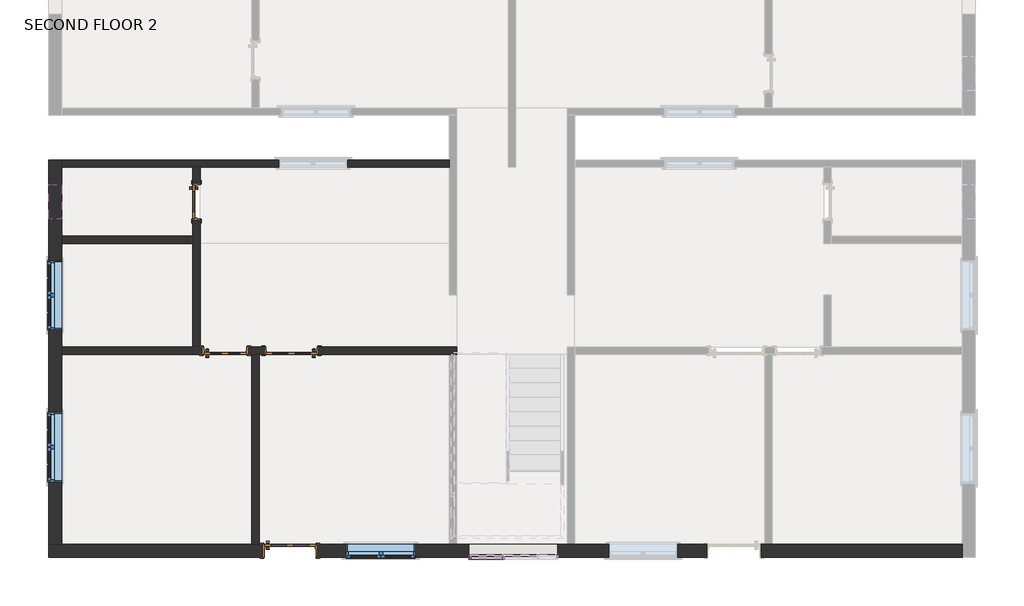
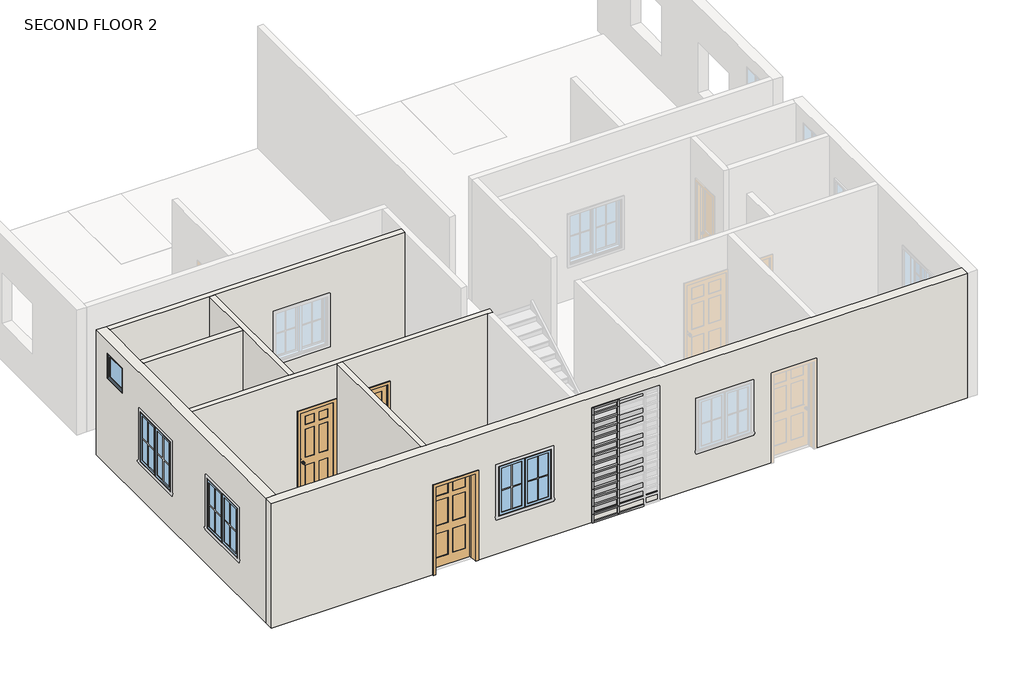
# One storey, part 1 of 4: 44 members, 21 plates, 7 walls, 4 doors, 4 windows.
"""IFC4 building model written with IfcOpenShell, lengths in millimetres."""

from ifc_helpers import new_model, si_unit, frame, origin, place, context, project, spatial, polyline, outline, extrude, faceted_brep, transform, mapped, element, save
from components import door_e337afa5, door_3b50870b, door_d86b6c54, door_03e3dfb5, member_56b223d9, member_a59c64b1, member_fa69921b, member_a67f877f, member_6a7c88b6, member_dc11c383, member_ff422208, system_panel_glazed_844a74e3, system_panel_glazed_a39216e9, system_panel_glazed_b3845325, system_panel_glazed_23b8b45c, system_panel_glazed_26c33eb0, system_panel_glazed_afc0885c, window_80340324, window_9200f5ac

model = new_model("IFC4")

# Units and contexts
model_context = context("Model", 3, world=origin())
ifc_project = project(units=[si_unit("LENGTHUNIT", "METRE", prefix="MILLI")], contexts=[model_context])

# Site, building, storey
site = spatial("IfcSite", under=ifc_project)
building = spatial("IfcBuilding", under=site)
storey = spatial("IfcBuildingStorey", under=building, Name="SECOND FLOOR 2", Elevation=6343.9725604)

# Doors
placement = place(None, origin())
door_shape = door_e337afa5(model_context)
element("IfcDoor", 1, ObjectType="Door-Interior-Single-2_Panel-Wood : 24\" x 84\"", at=placement, inside=storey, context=model_context, shape_type="MappedRepresentation", body=[
    mapped(door_shape, transform((-9830.0887331, -1548.6593836, 6343.9725604), x_axis=(0.0, -1.0, 0.0), y_axis=(1.0, 0.0, 0.0), z_axis=(0.0, 0.0, 1.0))),
])
door_2_shape = door_3b50870b(model_context)
element("IfcDoor", 2, ObjectType="Door-Interior-Single-6_Panel-Wood : 30\" x 84\"", at=placement, inside=storey, context=model_context, shape_type="MappedRepresentation", body=[
    mapped(door_2_shape, transform((-9318.9137331, -4180.7343836, 6343.9725604), x_axis=(1.0, 0.0, 0.0), y_axis=(0.0, 1.0, 0.0), z_axis=(0.0, 0.0, 1.0))),
])
door_3_shape = door_d86b6c54(model_context)
element("IfcDoor", 3, ObjectType="Door-Interior-Single-6_Panel-Wood : 36\" x 84\"", at=placement, inside=storey, context=model_context, shape_type="MappedRepresentation", body=[
    mapped(door_3_shape, transform((-8175.9137331, -7704.9843836, 6343.9725604), x_axis=(1.0, 0.0, 0.0), y_axis=(0.0, 1.0, 0.0), z_axis=(0.0, 0.0, 1.0))),
])
door_4_shape = door_03e3dfb5(model_context)
element("IfcDoor", 4, ObjectType="Door-Interior-Single-6_Panel-Wood : 36\" x 84\"", at=placement, inside=storey, context=model_context, shape_type="MappedRepresentation", body=[
    mapped(door_4_shape, transform((-8150.5137331, -4180.7343836, 6343.9725604), x_axis=(-1.0, 0.0, 0.0), y_axis=(0.0, -1.0, 0.0), z_axis=(0.0, 0.0, 1.0))),
])

# Members
member_shape = member_56b223d9(model_context)
element("IfcMember", 5, ObjectType="Rectangular Mullion : 1.5\" x 2.5\" rectangular", at=placement, inside=storey, context=model_context, shape_type="MappedRepresentation", body=[
    mapped(member_shape, transform((-4416.6334597, -7822.4593836, 6343.9725604), x_axis=(1.0, 0.0, 0.0), y_axis=(0.0, -1.0, 0.0), z_axis=(0.0, 0.0, -1.0))),
])
element("IfcMember", 6, ObjectType="Rectangular Mullion : 1.5\" x 2.5\" rectangular", at=placement, inside=storey, context=model_context, shape_type="MappedRepresentation", body=[
    mapped(member_shape, transform((-4416.6334597, -7822.4593836, 6547.1725604), x_axis=(1.0, 0.0, 0.0), y_axis=(0.0, -1.0, 0.0), z_axis=(0.0, 0.0, -1.0))),
])
element("IfcMember", 7, ObjectType="Rectangular Mullion : 1.5\" x 2.5\" rectangular", at=placement, inside=storey, context=model_context, shape_type="MappedRepresentation", body=[
    mapped(member_shape, transform((-4416.6334597, -7822.4593836, 6750.3725604), x_axis=(1.0, 0.0, 0.0), y_axis=(0.0, -1.0, 0.0), z_axis=(0.0, 0.0, -1.0))),
])
element("IfcMember", 8, ObjectType="Rectangular Mullion : 1.5\" x 2.5\" rectangular", at=placement, inside=storey, context=model_context, shape_type="MappedRepresentation", body=[
    mapped(member_shape, transform((-4416.6334597, -7822.4593836, 6953.5725604), x_axis=(1.0, 0.0, 0.0), y_axis=(0.0, -1.0, 0.0), z_axis=(0.0, 0.0, -1.0))),
])
element("IfcMember", 9, ObjectType="Rectangular Mullion : 1.5\" x 2.5\" rectangular", at=placement, inside=storey, context=model_context, shape_type="MappedRepresentation", body=[
    mapped(member_shape, transform((-4416.6334597, -7822.4593836, 7156.7725604), x_axis=(1.0, 0.0, 0.0), y_axis=(0.0, -1.0, 0.0), z_axis=(0.0, 0.0, -1.0))),
])
element("IfcMember", 10, ObjectType="Rectangular Mullion : 1.5\" x 2.5\" rectangular", at=placement, inside=storey, context=model_context, shape_type="MappedRepresentation", body=[
    mapped(member_shape, transform((-4416.6334597, -7822.4593836, 7359.9725604), x_axis=(1.0, 0.0, 0.0), y_axis=(0.0, -1.0, 0.0), z_axis=(0.0, 0.0, -1.0))),
])
element("IfcMember", 11, ObjectType="Rectangular Mullion : 1.5\" x 2.5\" rectangular", at=placement, inside=storey, context=model_context, shape_type="MappedRepresentation", body=[
    mapped(member_shape, transform((-4416.6334597, -7822.4593836, 7563.1725604), x_axis=(1.0, 0.0, 0.0), y_axis=(0.0, -1.0, 0.0), z_axis=(0.0, 0.0, -1.0))),
])
element("IfcMember", 12, ObjectType="Rectangular Mullion : 1.5\" x 2.5\" rectangular", at=placement, inside=storey, context=model_context, shape_type="MappedRepresentation", body=[
    mapped(member_shape, transform((-4416.6334597, -7822.4593836, 7766.3725604), x_axis=(1.0, 0.0, 0.0), y_axis=(0.0, -1.0, 0.0), z_axis=(0.0, 0.0, -1.0))),
])
element("IfcMember", 13, ObjectType="Rectangular Mullion : 1.5\" x 2.5\" rectangular", at=placement, inside=storey, context=model_context, shape_type="MappedRepresentation", body=[
    mapped(member_shape, transform((-4416.6334597, -7822.4593836, 7969.5725604), x_axis=(1.0, 0.0, 0.0), y_axis=(0.0, -1.0, 0.0), z_axis=(0.0, 0.0, -1.0))),
])
element("IfcMember", 14, ObjectType="Rectangular Mullion : 1.5\" x 2.5\" rectangular", at=placement, inside=storey, context=model_context, shape_type="MappedRepresentation", body=[
    mapped(member_shape, transform((-4416.6334597, -7822.4593836, 8172.7725604), x_axis=(1.0, 0.0, 0.0), y_axis=(0.0, -1.0, 0.0), z_axis=(0.0, 0.0, -1.0))),
])
element("IfcMember", 15, ObjectType="Rectangular Mullion : 1.5\" x 2.5\" rectangular", at=placement, inside=storey, context=model_context, shape_type="MappedRepresentation", body=[
    mapped(member_shape, transform((-4416.6334597, -7822.4593836, 8375.9725604), x_axis=(1.0, 0.0, 0.0), y_axis=(0.0, -1.0, 0.0), z_axis=(0.0, 0.0, -1.0))),
])
element("IfcMember", 16, ObjectType="Rectangular Mullion : 1.5\" x 2.5\" rectangular", at=placement, inside=storey, context=model_context, shape_type="MappedRepresentation", body=[
    mapped(member_shape, transform((-4416.6334597, -7822.4593836, 8579.1725604), x_axis=(1.0, 0.0, 0.0), y_axis=(0.0, -1.0, 0.0), z_axis=(0.0, 0.0, -1.0))),
])
element("IfcMember", 17, ObjectType="Rectangular Mullion : 1.5\" x 2.5\" rectangular", at=placement, inside=storey, context=model_context, shape_type="MappedRepresentation", body=[
    mapped(member_shape, transform((-4416.6334597, -7822.4593836, 8782.3725604), x_axis=(1.0, 0.0, 0.0), y_axis=(0.0, -1.0, 0.0), z_axis=(0.0, 0.0, -1.0))),
])
member_2_shape = member_a59c64b1(model_context)
element("IfcMember", 18, ObjectType="Rectangular Mullion : 1.5\" x 2.5\" rectangular", at=placement, inside=storey, context=model_context, shape_type="MappedRepresentation", body=[
    mapped(member_2_shape, transform((-4416.6334597, -7822.4593836, 8985.5725604), x_axis=(1.0, 0.0, 0.0), y_axis=(0.0, -1.0, 0.0), z_axis=(0.0, 0.0, -1.0))),
])
member_3_shape = member_fa69921b(model_context)
element("IfcMember", 19, ObjectType="Rectangular Mullion : 1.5\" x 2.5\" rectangular", at=placement, inside=storey, context=model_context, shape_type="MappedRepresentation", body=[
    mapped(member_3_shape, transform((-4435.6834597, -7822.4593836, 9151.3551755), x_axis=(0.0, 0.0, 1.0), y_axis=(0.0, -1.0, 0.0), z_axis=(1.0, 0.0, 0.0))),
])
element("IfcMember", 20, ObjectType="Rectangular Mullion : 1.5\" x 2.5\" rectangular", at=placement, inside=storey, context=model_context, shape_type="MappedRepresentation", body=[
    mapped(member_3_shape, transform((-4988.13346, -7822.4593836, 6343.9725604), x_axis=(0.0, 0.0, -1.0), y_axis=(0.0, -1.0, 0.0), z_axis=(-1.0, 0.0, 0.0))),
])
member_4_shape = member_a67f877f(model_context)
element("IfcMember", 21, ObjectType="Rectangular Mullion : 1.5\" x 2.5\" rectangular", at=placement, inside=storey, context=model_context, shape_type="MappedRepresentation", body=[
    mapped(member_4_shape, transform((-4397.5834597, -7822.4593836, 6343.9725604), x_axis=(0.0, 0.0, -1.0), y_axis=(0.0, -1.0, 0.0), z_axis=(-1.0, 0.0, 0.0))),
])
member_5_shape = member_6a7c88b6(model_context)
element("IfcMember", 22, ObjectType="Rectangular Mullion : 1.5\" x 2.5\" rectangular", at=placement, inside=storey, context=model_context, shape_type="MappedRepresentation", body=[
    mapped(member_5_shape, transform((-4435.6834597, -7822.4593836, 6547.1725604), x_axis=(0.0, 0.0, 1.0), y_axis=(0.0, -1.0, 0.0), z_axis=(1.0, 0.0, 0.0))),
])
element("IfcMember", 23, ObjectType="Rectangular Mullion : 1.5\" x 2.5\" rectangular", at=placement, inside=storey, context=model_context, shape_type="MappedRepresentation", body=[
    mapped(member_5_shape, transform((-4435.6834597, -7822.4593836, 6750.3725604), x_axis=(0.0, 0.0, 1.0), y_axis=(0.0, -1.0, 0.0), z_axis=(1.0, 0.0, 0.0))),
])
element("IfcMember", 24, ObjectType="Rectangular Mullion : 1.5\" x 2.5\" rectangular", at=placement, inside=storey, context=model_context, shape_type="MappedRepresentation", body=[
    mapped(member_5_shape, transform((-4435.6834597, -7822.4593836, 6953.5725604), x_axis=(0.0, 0.0, 1.0), y_axis=(0.0, -1.0, 0.0), z_axis=(1.0, 0.0, 0.0))),
])
element("IfcMember", 25, ObjectType="Rectangular Mullion : 1.5\" x 2.5\" rectangular", at=placement, inside=storey, context=model_context, shape_type="MappedRepresentation", body=[
    mapped(member_5_shape, transform((-4435.6834597, -7822.4593836, 7156.7725604), x_axis=(0.0, 0.0, 1.0), y_axis=(0.0, -1.0, 0.0), z_axis=(1.0, 0.0, 0.0))),
])
element("IfcMember", 26, ObjectType="Rectangular Mullion : 1.5\" x 2.5\" rectangular", at=placement, inside=storey, context=model_context, shape_type="MappedRepresentation", body=[
    mapped(member_5_shape, transform((-4435.6834597, -7822.4593836, 7359.9725604), x_axis=(0.0, 0.0, 1.0), y_axis=(0.0, -1.0, 0.0), z_axis=(1.0, 0.0, 0.0))),
])
element("IfcMember", 27, ObjectType="Rectangular Mullion : 1.5\" x 2.5\" rectangular", at=placement, inside=storey, context=model_context, shape_type="MappedRepresentation", body=[
    mapped(member_5_shape, transform((-4435.6834597, -7822.4593836, 7563.1725604), x_axis=(0.0, 0.0, 1.0), y_axis=(0.0, -1.0, 0.0), z_axis=(1.0, 0.0, 0.0))),
])
element("IfcMember", 28, ObjectType="Rectangular Mullion : 1.5\" x 2.5\" rectangular", at=placement, inside=storey, context=model_context, shape_type="MappedRepresentation", body=[
    mapped(member_5_shape, transform((-4435.6834597, -7822.4593836, 7766.3725604), x_axis=(0.0, 0.0, 1.0), y_axis=(0.0, -1.0, 0.0), z_axis=(1.0, 0.0, 0.0))),
])
element("IfcMember", 29, ObjectType="Rectangular Mullion : 1.5\" x 2.5\" rectangular", at=placement, inside=storey, context=model_context, shape_type="MappedRepresentation", body=[
    mapped(member_5_shape, transform((-4435.6834597, -7822.4593836, 7969.5725604), x_axis=(0.0, 0.0, 1.0), y_axis=(0.0, -1.0, 0.0), z_axis=(1.0, 0.0, 0.0))),
])
element("IfcMember", 30, ObjectType="Rectangular Mullion : 1.5\" x 2.5\" rectangular", at=placement, inside=storey, context=model_context, shape_type="MappedRepresentation", body=[
    mapped(member_5_shape, transform((-4435.6834597, -7822.4593836, 8172.7725604), x_axis=(0.0, 0.0, 1.0), y_axis=(0.0, -1.0, 0.0), z_axis=(1.0, 0.0, 0.0))),
])
element("IfcMember", 31, ObjectType="Rectangular Mullion : 1.5\" x 2.5\" rectangular", at=placement, inside=storey, context=model_context, shape_type="MappedRepresentation", body=[
    mapped(member_5_shape, transform((-4435.6834597, -7822.4593836, 8375.9725604), x_axis=(0.0, 0.0, 1.0), y_axis=(0.0, -1.0, 0.0), z_axis=(1.0, 0.0, 0.0))),
])
element("IfcMember", 32, ObjectType="Rectangular Mullion : 1.5\" x 2.5\" rectangular", at=placement, inside=storey, context=model_context, shape_type="MappedRepresentation", body=[
    mapped(member_5_shape, transform((-4435.6834597, -7822.4593836, 8579.1725604), x_axis=(0.0, 0.0, 1.0), y_axis=(0.0, -1.0, 0.0), z_axis=(1.0, 0.0, 0.0))),
])
element("IfcMember", 33, ObjectType="Rectangular Mullion : 1.5\" x 2.5\" rectangular", at=placement, inside=storey, context=model_context, shape_type="MappedRepresentation", body=[
    mapped(member_5_shape, transform((-4435.6834597, -7822.4593836, 8782.3725604), x_axis=(0.0, 0.0, 1.0), y_axis=(0.0, -1.0, 0.0), z_axis=(1.0, 0.0, 0.0))),
])
element("IfcMember", 34, ObjectType="Rectangular Mullion : 1.5\" x 2.5\" rectangular", at=placement, inside=storey, context=model_context, shape_type="MappedRepresentation", body=[
    mapped(member_5_shape, transform((-4435.6834597, -7822.4593836, 8985.5725604), x_axis=(0.0, 0.0, 1.0), y_axis=(0.0, -1.0, 0.0), z_axis=(1.0, 0.0, 0.0))),
])
member_6_shape = member_dc11c383(model_context)
element("IfcMember", 35, ObjectType="Rectangular Mullion : 1.5\" x 2.5\" rectangular", at=placement, inside=storey, context=model_context, shape_type="MappedRepresentation", body=[
    mapped(member_6_shape, transform((-5026.23346, -7822.4593836, 9151.3551755), x_axis=(-1.0, 0.0, 0.0), y_axis=(0.0, -1.0, 0.0), z_axis=(0.0, 0.0, 1.0))),
])
member_7_shape = member_ff422208(model_context)
element("IfcMember", 36, ObjectType="Rectangular Mullion : 1.5\" x 2.5\" rectangular", at=placement, inside=storey, context=model_context, shape_type="MappedRepresentation", body=[
    mapped(member_7_shape, transform((-5026.23346, -7822.4593836, 6547.1725604), x_axis=(-1.0, 0.0, 0.0), y_axis=(0.0, -1.0, 0.0), z_axis=(0.0, 0.0, 1.0))),
])
element("IfcMember", 37, ObjectType="Rectangular Mullion : 1.5\" x 2.5\" rectangular", at=placement, inside=storey, context=model_context, shape_type="MappedRepresentation", body=[
    mapped(member_7_shape, transform((-5026.23346, -7822.4593836, 6750.3725604), x_axis=(-1.0, 0.0, 0.0), y_axis=(0.0, -1.0, 0.0), z_axis=(0.0, 0.0, 1.0))),
])
element("IfcMember", 38, ObjectType="Rectangular Mullion : 1.5\" x 2.5\" rectangular", at=placement, inside=storey, context=model_context, shape_type="MappedRepresentation", body=[
    mapped(member_7_shape, transform((-5026.23346, -7822.4593836, 6953.5725604), x_axis=(-1.0, 0.0, 0.0), y_axis=(0.0, -1.0, 0.0), z_axis=(0.0, 0.0, 1.0))),
])
element("IfcMember", 39, ObjectType="Rectangular Mullion : 1.5\" x 2.5\" rectangular", at=placement, inside=storey, context=model_context, shape_type="MappedRepresentation", body=[
    mapped(member_7_shape, transform((-5026.23346, -7822.4593836, 7156.7725604), x_axis=(-1.0, 0.0, 0.0), y_axis=(0.0, -1.0, 0.0), z_axis=(0.0, 0.0, 1.0))),
])
element("IfcMember", 40, ObjectType="Rectangular Mullion : 1.5\" x 2.5\" rectangular", at=placement, inside=storey, context=model_context, shape_type="MappedRepresentation", body=[
    mapped(member_7_shape, transform((-5026.23346, -7822.4593836, 7359.9725604), x_axis=(-1.0, 0.0, 0.0), y_axis=(0.0, -1.0, 0.0), z_axis=(0.0, 0.0, 1.0))),
])
element("IfcMember", 41, ObjectType="Rectangular Mullion : 1.5\" x 2.5\" rectangular", at=placement, inside=storey, context=model_context, shape_type="MappedRepresentation", body=[
    mapped(member_7_shape, transform((-5026.23346, -7822.4593836, 7563.1725604), x_axis=(-1.0, 0.0, 0.0), y_axis=(0.0, -1.0, 0.0), z_axis=(0.0, 0.0, 1.0))),
])
element("IfcMember", 42, ObjectType="Rectangular Mullion : 1.5\" x 2.5\" rectangular", at=placement, inside=storey, context=model_context, shape_type="MappedRepresentation", body=[
    mapped(member_7_shape, transform((-5026.23346, -7822.4593836, 7766.3725604), x_axis=(-1.0, 0.0, 0.0), y_axis=(0.0, -1.0, 0.0), z_axis=(0.0, 0.0, 1.0))),
])
element("IfcMember", 43, ObjectType="Rectangular Mullion : 1.5\" x 2.5\" rectangular", at=placement, inside=storey, context=model_context, shape_type="MappedRepresentation", body=[
    mapped(member_7_shape, transform((-5026.23346, -7822.4593836, 7969.5725604), x_axis=(-1.0, 0.0, 0.0), y_axis=(0.0, -1.0, 0.0), z_axis=(0.0, 0.0, 1.0))),
])
element("IfcMember", 44, ObjectType="Rectangular Mullion : 1.5\" x 2.5\" rectangular", at=placement, inside=storey, context=model_context, shape_type="MappedRepresentation", body=[
    mapped(member_7_shape, transform((-5026.23346, -7822.4593836, 8172.7725604), x_axis=(-1.0, 0.0, 0.0), y_axis=(0.0, -1.0, 0.0), z_axis=(0.0, 0.0, 1.0))),
])
element("IfcMember", 45, ObjectType="Rectangular Mullion : 1.5\" x 2.5\" rectangular", at=placement, inside=storey, context=model_context, shape_type="MappedRepresentation", body=[
    mapped(member_7_shape, transform((-5026.23346, -7822.4593836, 8375.9725604), x_axis=(-1.0, 0.0, 0.0), y_axis=(0.0, -1.0, 0.0), z_axis=(0.0, 0.0, 1.0))),
])
element("IfcMember", 46, ObjectType="Rectangular Mullion : 1.5\" x 2.5\" rectangular", at=placement, inside=storey, context=model_context, shape_type="MappedRepresentation", body=[
    mapped(member_7_shape, transform((-5026.23346, -7822.4593836, 8579.1725604), x_axis=(-1.0, 0.0, 0.0), y_axis=(0.0, -1.0, 0.0), z_axis=(0.0, 0.0, 1.0))),
])
element("IfcMember", 47, ObjectType="Rectangular Mullion : 1.5\" x 2.5\" rectangular", at=placement, inside=storey, context=model_context, shape_type="MappedRepresentation", body=[
    mapped(member_7_shape, transform((-5026.23346, -7822.4593836, 8782.3725604), x_axis=(-1.0, 0.0, 0.0), y_axis=(0.0, -1.0, 0.0), z_axis=(0.0, 0.0, 1.0))),
])
element("IfcMember", 48, ObjectType="Rectangular Mullion : 1.5\" x 2.5\" rectangular", at=placement, inside=storey, context=model_context, shape_type="MappedRepresentation", body=[
    mapped(member_7_shape, transform((-5026.23346, -7822.4593836, 8985.5725604), x_axis=(-1.0, 0.0, 0.0), y_axis=(0.0, -1.0, 0.0), z_axis=(0.0, 0.0, 1.0))),
])

# Plates
system_panel_glazed_shape = system_panel_glazed_844a74e3(model_context)
element("IfcPlate", 49, ObjectType="System Panel : Glazed", at=placement, inside=storey, context=model_context, shape_type="MappedRepresentation", body=[
    mapped(system_panel_glazed_shape, transform((-4711.9084599, -7822.4593836, 6382.0725604), x_axis=(1.0, 0.0, 0.0), y_axis=(0.0, 1.0, 0.0), z_axis=(0.0, 0.0, 1.0))),
])
system_panel_glazed_2_shape = system_panel_glazed_a39216e9(model_context)
element("IfcPlate", 50, ObjectType="System Panel : Glazed", at=placement, inside=storey, context=model_context, shape_type="MappedRepresentation", body=[
    mapped(system_panel_glazed_2_shape, transform((-4111.8334597, -7822.4593836, 6382.0725604), x_axis=(1.0, 0.0, 0.0), y_axis=(0.0, 1.0, 0.0), z_axis=(0.0, 0.0, 1.0))),
])
system_panel_glazed_3_shape = system_panel_glazed_b3845325(model_context)
element("IfcPlate", 51, ObjectType="System Panel : Glazed", at=placement, inside=storey, context=model_context, shape_type="MappedRepresentation", body=[
    mapped(system_panel_glazed_3_shape, transform((-4711.9084599, -7822.4593836, 6566.2225604), x_axis=(1.0, 0.0, 0.0), y_axis=(0.0, 1.0, 0.0), z_axis=(0.0, 0.0, 1.0))),
])
element("IfcPlate", 52, ObjectType="System Panel : Glazed", at=placement, inside=storey, context=model_context, shape_type="MappedRepresentation", body=[
    mapped(system_panel_glazed_3_shape, transform((-4711.9084599, -7822.4593836, 6769.4225604), x_axis=(1.0, 0.0, 0.0), y_axis=(0.0, 1.0, 0.0), z_axis=(0.0, 0.0, 1.0))),
])
element("IfcPlate", 53, ObjectType="System Panel : Glazed", at=placement, inside=storey, context=model_context, shape_type="MappedRepresentation", body=[
    mapped(system_panel_glazed_3_shape, transform((-4711.9084599, -7822.4593836, 7175.8225604), x_axis=(1.0, 0.0, 0.0), y_axis=(0.0, 1.0, 0.0), z_axis=(0.0, 0.0, 1.0))),
])
element("IfcPlate", 54, ObjectType="System Panel : Glazed", at=placement, inside=storey, context=model_context, shape_type="MappedRepresentation", body=[
    mapped(system_panel_glazed_3_shape, transform((-4711.9084599, -7822.4593836, 7379.0225604), x_axis=(1.0, 0.0, 0.0), y_axis=(0.0, 1.0, 0.0), z_axis=(0.0, 0.0, 1.0))),
])
element("IfcPlate", 55, ObjectType="System Panel : Glazed", at=placement, inside=storey, context=model_context, shape_type="MappedRepresentation", body=[
    mapped(system_panel_glazed_3_shape, transform((-4711.9084599, -7822.4593836, 7785.4225604), x_axis=(1.0, 0.0, 0.0), y_axis=(0.0, 1.0, 0.0), z_axis=(0.0, 0.0, 1.0))),
])
element("IfcPlate", 56, ObjectType="System Panel : Glazed", at=placement, inside=storey, context=model_context, shape_type="MappedRepresentation", body=[
    mapped(system_panel_glazed_3_shape, transform((-4711.9084599, -7822.4593836, 7988.6225604), x_axis=(1.0, 0.0, 0.0), y_axis=(0.0, 1.0, 0.0), z_axis=(0.0, 0.0, 1.0))),
])
element("IfcPlate", 57, ObjectType="System Panel : Glazed", at=placement, inside=storey, context=model_context, shape_type="MappedRepresentation", body=[
    mapped(system_panel_glazed_3_shape, transform((-4711.9084599, -7822.4593836, 8395.0225604), x_axis=(1.0, 0.0, 0.0), y_axis=(0.0, 1.0, 0.0), z_axis=(0.0, 0.0, 1.0))),
])
element("IfcPlate", 58, ObjectType="System Panel : Glazed", at=placement, inside=storey, context=model_context, shape_type="MappedRepresentation", body=[
    mapped(system_panel_glazed_3_shape, transform((-4711.9084599, -7822.4593836, 8598.2225604), x_axis=(1.0, 0.0, 0.0), y_axis=(0.0, 1.0, 0.0), z_axis=(0.0, 0.0, 1.0))),
])
element("IfcPlate", 59, ObjectType="System Panel : Glazed", at=placement, inside=storey, context=model_context, shape_type="MappedRepresentation", body=[
    mapped(system_panel_glazed_3_shape, transform((-4711.9084599, -7822.4593836, 6972.6225604), x_axis=(1.0, 0.0, 0.0), y_axis=(0.0, 1.0, 0.0), z_axis=(0.0, 0.0, 1.0))),
])
system_panel_glazed_4_shape = system_panel_glazed_23b8b45c(model_context)
element("IfcPlate", 60, ObjectType="System Panel : Glazed", at=placement, inside=storey, context=model_context, shape_type="MappedRepresentation", body=[
    mapped(system_panel_glazed_4_shape, transform((-4111.8334597, -7822.4593836, 6566.2225604), x_axis=(1.0, 0.0, 0.0), y_axis=(0.0, 1.0, 0.0), z_axis=(0.0, 0.0, 1.0))),
])
element("IfcPlate", 61, ObjectType="System Panel : Glazed", at=placement, inside=storey, context=model_context, shape_type="MappedRepresentation", body=[
    mapped(system_panel_glazed_4_shape, transform((-4111.8334597, -7822.4593836, 6769.4225604), x_axis=(1.0, 0.0, 0.0), y_axis=(0.0, 1.0, 0.0), z_axis=(0.0, 0.0, 1.0))),
])
element("IfcPlate", 62, ObjectType="System Panel : Glazed", at=placement, inside=storey, context=model_context, shape_type="MappedRepresentation", body=[
    mapped(system_panel_glazed_4_shape, transform((-4111.8334597, -7822.4593836, 7175.8225604), x_axis=(1.0, 0.0, 0.0), y_axis=(0.0, 1.0, 0.0), z_axis=(0.0, 0.0, 1.0))),
])
element("IfcPlate", 63, ObjectType="System Panel : Glazed", at=placement, inside=storey, context=model_context, shape_type="MappedRepresentation", body=[
    mapped(system_panel_glazed_4_shape, transform((-4111.8334597, -7822.4593836, 7379.0225604), x_axis=(1.0, 0.0, 0.0), y_axis=(0.0, 1.0, 0.0), z_axis=(0.0, 0.0, 1.0))),
])
element("IfcPlate", 64, ObjectType="System Panel : Glazed", at=placement, inside=storey, context=model_context, shape_type="MappedRepresentation", body=[
    mapped(system_panel_glazed_4_shape, transform((-4111.8334597, -7822.4593836, 7785.4225604), x_axis=(1.0, 0.0, 0.0), y_axis=(0.0, 1.0, 0.0), z_axis=(0.0, 0.0, 1.0))),
])
element("IfcPlate", 65, ObjectType="System Panel : Glazed", at=placement, inside=storey, context=model_context, shape_type="MappedRepresentation", body=[
    mapped(system_panel_glazed_4_shape, transform((-4111.8334597, -7822.4593836, 7988.6225604), x_axis=(1.0, 0.0, 0.0), y_axis=(0.0, 1.0, 0.0), z_axis=(0.0, 0.0, 1.0))),
])
element("IfcPlate", 66, ObjectType="System Panel : Glazed", at=placement, inside=storey, context=model_context, shape_type="MappedRepresentation", body=[
    mapped(system_panel_glazed_4_shape, transform((-4111.8334597, -7822.4593836, 8395.0225604), x_axis=(1.0, 0.0, 0.0), y_axis=(0.0, 1.0, 0.0), z_axis=(0.0, 0.0, 1.0))),
])
element("IfcPlate", 67, ObjectType="System Panel : Glazed", at=placement, inside=storey, context=model_context, shape_type="MappedRepresentation", body=[
    mapped(system_panel_glazed_4_shape, transform((-4111.8334597, -7822.4593836, 8598.2225604), x_axis=(1.0, 0.0, 0.0), y_axis=(0.0, 1.0, 0.0), z_axis=(0.0, 0.0, 1.0))),
])
system_panel_glazed_5_shape = system_panel_glazed_26c33eb0(model_context)
element("IfcPlate", 68, ObjectType="System Panel : Glazed", at=placement, inside=storey, context=model_context, shape_type="MappedRepresentation", body=[
    mapped(system_panel_glazed_5_shape, transform((-4711.9084599, -7822.4593836, 9004.6225604), x_axis=(1.0, 0.0, 0.0), y_axis=(0.0, 1.0, 0.0), z_axis=(0.0, 0.0, 1.0))),
])
system_panel_glazed_6_shape = system_panel_glazed_afc0885c(model_context)
element("IfcPlate", 69, ObjectType="System Panel : Glazed", at=placement, inside=storey, context=model_context, shape_type="MappedRepresentation", body=[
    mapped(system_panel_glazed_6_shape, transform((-4111.8334597, -7822.4593836, 9004.6225604), x_axis=(1.0, 0.0, 0.0), y_axis=(0.0, 1.0, 0.0), z_axis=(0.0, 0.0, 1.0))),
])

# Walls
element("IfcWall", 70, ObjectType="Inner Wall 5\"", at=placement, inside=storey, context=model_context, shape_type="Brep", body=[
    faceted_brep([(-12201.8137331, -939.0593836, 6343.9725604), (-9890.4137331, -939.0593836, 6343.9725604), (-9763.4137331, -939.0593836, 6343.9725604), (-5369.2137331, -939.0593836, 6343.9725604), (-5369.2137331, -939.0593836, 9391.9725604), (-9763.4137331, -939.0593836, 9391.9725604), (-9890.4137331, -939.0593836, 9391.9725604), (-12201.8137331, -939.0593836, 9391.9725604), (-7159.9137331, -939.0593836, 8477.5725604), (-7159.9137331, -939.0593836, 7258.3725604), (-8379.1137331, -939.0593836, 7258.3725604), (-8379.1137331, -939.0593836, 8477.5725604), (-12201.8137331, -812.0593836, 6343.9725604), (-12201.8137331, -812.0593836, 9391.9725604), (-5369.2137331, -812.0593836, 9391.9725604), (-5369.2137331, -812.0593836, 6343.9725604), (-7159.9137331, -812.0593836, 8477.5725604), (-8379.1137331, -812.0593836, 8477.5725604), (-8379.1137331, -812.0593836, 7258.3725604), (-7159.9137331, -812.0593836, 7258.3725604)], [[[0, 1, 2, 3, 4, 5, 6, 7], [8, 9, 10, 11]], [[12, 13, 14, 15], [16, 17, 18, 19]], [[3, 2, 1, 0, 12, 15]], [[7, 6, 5, 4, 14, 13]], [[0, 7, 13, 12]], [[4, 3, 15, 14]], [[9, 8, 16, 19]], [[10, 9, 19, 18]], [[11, 10, 18, 17]], [[8, 11, 17, 16]]]),
])
element("IfcWall", 71, ObjectType="Inner Wall 5\"", at=placement, inside=storey, context=model_context, shape_type="SweptSolid", body=[
    extrude(outline(polyline([(-8722.0137331, -4241.0593836), (-8722.0137331, -7593.8593836), (-8849.0137331, -7593.8593836), (-8849.0137331, -4241.0593836), (-8722.0137331, -4241.0593836)])), frame((0.0, 0.0, 6343.9725604), z_axis=(0.0, 0.0, 1.0), x_axis=(1.0, 0.0, 0.0)), (0.0, 0.0, 1.0), 3048.0),
])
element("IfcWall", 72, ObjectType="Inner Wall 5\"", at=placement, inside=storey, context=model_context, shape_type="Brep", body=[
    faceted_brep([(-12201.8137331, -4114.0593836, 9391.9725604), (-9890.4137331, -4114.0593836, 9391.9725604), (-9763.4137331, -4114.0593836, 9391.9725604), (-5242.2137331, -4114.0593836, 9391.9725604), (-5242.2137331, -4114.0593836, 6343.9725604), (-7667.9137331, -4114.0593836, 6343.9725604), (-7667.9137331, -4114.0593836, 8502.9725604), (-8633.1137331, -4114.0593836, 8502.9725604), (-8633.1137331, -4114.0593836, 6343.9725604), (-8912.5137331, -4114.0593836, 6343.9725604), (-8912.5137331, -4114.0593836, 8502.9725604), (-9725.3137331, -4114.0593836, 8502.9725604), (-9725.3137331, -4114.0593836, 6343.9725604), (-9763.4137331, -4114.0593836, 6343.9725604), (-9890.4137331, -4114.0593836, 6343.9725604), (-12201.8137331, -4114.0593836, 6343.9725604), (-5242.2137331, -4241.0593836, 9391.9725604), (-5369.2137331, -4241.0593836, 9391.9725604), (-8722.0137331, -4241.0593836, 9391.9725604), (-8849.0137331, -4241.0593836, 9391.9725604), (-12201.8137331, -4241.0593836, 9391.9725604), (-12201.8137331, -4241.0593836, 6343.9725604), (-9725.3137331, -4241.0593836, 6343.9725604), (-9725.3137331, -4241.0593836, 8502.9725604), (-8912.5137331, -4241.0593836, 8502.9725604), (-8912.5137331, -4241.0593836, 6343.9725604), (-8849.0137331, -4241.0593836, 6343.9725604), (-8722.0137331, -4241.0593836, 6343.9725604), (-8633.1137331, -4241.0593836, 6343.9725604), (-8633.1137331, -4241.0593836, 8502.9725604), (-7667.9137331, -4241.0593836, 8502.9725604), (-7667.9137331, -4241.0593836, 6343.9725604), (-5369.2137331, -4241.0593836, 6343.9725604), (-5242.2137331, -4241.0593836, 6343.9725604)], [[[0, 1, 2, 3, 4, 5, 6, 7, 8, 9, 10, 11, 12, 13, 14, 15]], [[16, 17, 18, 19, 20, 21, 22, 23, 24, 25, 26, 27, 28, 29, 30, 31, 32, 33]], [[21, 15, 14, 13, 12, 22]], [[4, 33, 32, 31, 5]], [[25, 9, 8, 28, 27, 26]], [[3, 2, 1, 0, 20, 19, 18, 17, 16]], [[0, 15, 21, 20]], [[4, 3, 16, 33]], [[10, 9, 25, 24]], [[11, 10, 24, 23]], [[12, 11, 23, 22]], [[7, 29, 28, 8]], [[29, 7, 6, 30]], [[30, 6, 5, 31]]]),
])
element("IfcWall", 73, ObjectType="Inner Wall 5\"", at=placement, inside=storey, context=model_context, shape_type="Brep", body=[
    faceted_brep([(-9763.4137331, -939.0593836, 9391.9725604), (-9763.4137331, -4114.0593836, 9391.9725604), (-9763.4137331, -4114.0593836, 6343.9725604), (-9763.4137331, -1878.8593836, 6343.9725604), (-9763.4137331, -1878.8593836, 8502.9725604), (-9763.4137331, -1218.4593836, 8502.9725604), (-9763.4137331, -1218.4593836, 6343.9725604), (-9763.4137331, -939.0593836, 6343.9725604), (-9890.4137331, -4114.0593836, 9391.9725604), (-9890.4137331, -2285.2593836, 9391.9725604), (-9890.4137331, -2158.2593836, 9391.9725604), (-9890.4137331, -939.0593836, 9391.9725604), (-9890.4137331, -939.0593836, 6343.9725604), (-9890.4137331, -1218.4593836, 6343.9725604), (-9890.4137331, -1218.4593836, 8502.9725604), (-9890.4137331, -1878.8593836, 8502.9725604), (-9890.4137331, -1878.8593836, 6343.9725604), (-9890.4137331, -2158.2593836, 6343.9725604), (-9890.4137331, -2285.2593836, 6343.9725604), (-9890.4137331, -4114.0593836, 6343.9725604)], [[[0, 1, 2, 3, 4, 5, 6, 7]], [[8, 9, 10, 11, 12, 13, 14, 15, 16, 17, 18, 19]], [[2, 19, 18, 17, 16, 3]], [[12, 7, 6, 13]], [[1, 0, 11, 10, 9, 8]], [[2, 1, 8, 19]], [[0, 7, 12, 11]], [[15, 4, 3, 16]], [[4, 15, 14, 5]], [[5, 14, 13, 6]]]),
])
element("IfcWall", 74, ObjectType="Inner Wall 5\"", at=placement, inside=storey, context=model_context, shape_type="SweptSolid", body=[
    extrude(outline(polyline([(-12201.8137331, -2158.2593836), (-9890.4137331, -2158.2593836), (-9890.4137331, -2285.2593836), (-12201.8137331, -2285.2593836), (-12201.8137331, -2158.2593836)])), frame((0.0, 0.0, 6343.9725604), z_axis=(0.0, 0.0, 1.0), x_axis=(1.0, 0.0, 0.0)), (0.0, 0.0, 1.0), 3048.0),
])
element("IfcWall", 75, ObjectType="outer wall 9\"", at=placement, inside=storey, context=model_context, shape_type="Brep", body=[
    faceted_brep([(3673.1862669, -7822.4593836, 9391.9725604), (-12430.4137331, -7822.4593836, 9391.9725604), (-12430.4137331, -7822.4593836, 6343.9725604), (-8658.5137331, -7822.4593836, 6343.9725604), (-8658.5137331, -7822.4593836, 8502.9725604), (-7693.3137331, -7822.4593836, 8502.9725604), (-7693.3137331, -7822.4593836, 6343.9725604), (-835.3137331, -7822.4593836, 6343.9725604), (-835.3137331, -7822.4593836, 8502.9725604), (129.8862669, -7822.4593836, 8502.9725604), (129.8862669, -7822.4593836, 6343.9725604), (3673.1862669, -7822.4593836, 6343.9725604), (-2562.5137331, -7822.4593836, 8477.5725604), (-1343.3137331, -7822.4593836, 8477.5725604), (-1343.3137331, -7822.4593836, 7258.3725604), (-2562.5137331, -7822.4593836, 7258.3725604), (-7185.3137331, -7822.4593836, 8477.5725604), (-5966.1137331, -7822.4593836, 8477.5725604), (-5966.1137331, -7822.4593836, 7258.3725604), (-7185.3137331, -7822.4593836, 7258.3725604), (-5026.23346, -7822.4593836, 9151.3551755), (-3461.6513929, -7822.4593836, 9151.3551755), (-3461.6513929, -7822.4593836, 6578.4868874), (-5026.23346, -7822.4593836, 6578.4868874), (-12430.4137331, -7593.8593836, 9391.9725604), (-12201.8137331, -7593.8593836, 9391.9725604), (-8849.0137331, -7593.8593836, 9391.9725604), (-8722.0137331, -7593.8593836, 9391.9725604), (-5369.2137331, -7593.8593836, 9391.9725604), (-5242.2137331, -7593.8593836, 9391.9725604), (-3286.4137331, -7593.8593836, 9391.9725604), (-3159.4137331, -7593.8593836, 9391.9725604), (193.3862669, -7593.8593836, 9391.9725604), (320.3862669, -7593.8593836, 9391.9725604), (3673.1862669, -7593.8593836, 9391.9725604), (3673.1862669, -7593.8593836, 6343.9725604), (320.3862669, -7593.8593836, 6343.9725604), (193.3862669, -7593.8593836, 6343.9725604), (129.8862669, -7593.8593836, 6343.9725604), (129.8862669, -7593.8593836, 8502.9725604), (-835.3137331, -7593.8593836, 8502.9725604), (-835.3137331, -7593.8593836, 6343.9725604), (-3159.4137331, -7593.8593836, 6343.9725604), (-3286.4137331, -7593.8593836, 6343.9725604), (-5242.2137331, -7593.8593836, 6343.9725604), (-5369.2137331, -7593.8593836, 6343.9725604), (-7693.3137331, -7593.8593836, 6343.9725604), (-7693.3137331, -7593.8593836, 8502.9725604), (-8658.5137331, -7593.8593836, 8502.9725604), (-8658.5137331, -7593.8593836, 6343.9725604), (-8722.0137331, -7593.8593836, 6343.9725604), (-8849.0137331, -7593.8593836, 6343.9725604), (-12201.8137331, -7593.8593836, 6343.9725604), (-12430.4137331, -7593.8593836, 6343.9725604), (-2562.5137331, -7593.8593836, 8477.5725604), (-2562.5137331, -7593.8593836, 7258.3725604), (-1343.3137331, -7593.8593836, 7258.3725604), (-1343.3137331, -7593.8593836, 8477.5725604), (-7185.3137331, -7593.8593836, 8477.5725604), (-7185.3137331, -7593.8593836, 7258.3725604), (-5966.1137331, -7593.8593836, 7258.3725604), (-5966.1137331, -7593.8593836, 8477.5725604), (-3461.6513929, -7593.8593836, 9151.3551755), (-5026.23346, -7593.8593836, 9151.3551755), (-5026.23346, -7593.8593836, 6578.4868874), (-3461.6513929, -7593.8593836, 6578.4868874)], [[[0, 1, 2, 3, 4, 5, 6, 7, 8, 9, 10, 11], [12, 13, 14, 15], [16, 17, 18, 19], [20, 21, 22, 23]], [[24, 25, 26, 27, 28, 29, 30, 31, 32, 33, 34, 35, 36, 37, 38, 39, 40, 41, 42, 43, 44, 45, 46, 47, 48, 49, 50, 51, 52, 53], [54, 55, 56, 57], [58, 59, 60, 61], [62, 63, 64, 65]], [[2, 53, 52, 51, 50, 49, 3]], [[35, 11, 10, 38, 37, 36]], [[6, 46, 45, 44, 43, 42, 41, 7]], [[1, 0, 34, 33, 32, 31, 30, 29, 28, 27, 26, 25, 24]], [[2, 1, 24, 53]], [[0, 11, 35, 34]], [[5, 47, 46, 6]], [[47, 5, 4, 48]], [[48, 4, 3, 49]], [[40, 8, 7, 41]], [[8, 40, 39, 9]], [[9, 39, 38, 10]], [[55, 54, 12, 15]], [[56, 55, 15, 14]], [[57, 56, 14, 13]], [[54, 57, 13, 12]], [[59, 58, 16, 19]], [[60, 59, 19, 18]], [[61, 60, 18, 17]], [[58, 61, 17, 16]], [[20, 63, 62, 21]], [[22, 65, 64, 23]], [[63, 20, 23, 64]], [[21, 62, 65, 22]]]),
])
element("IfcWall", 76, ObjectType="outer wall 9\"", at=placement, inside=storey, context=model_context, shape_type="Brep", body=[
    faceted_brep([(-12430.4137331, -812.0593836, 6343.9725604), (-12430.4137331, -7593.8593836, 6343.9725604), (-12430.4137331, -7593.8593836, 9391.9725604), (-12430.4137331, -812.0593836, 9391.9725604), (-12430.4137331, -5269.7593836, 8477.5725604), (-12430.4137331, -6488.9593836, 8477.5725604), (-12430.4137331, -6488.9593836, 7258.3725604), (-12430.4137331, -5269.7593836, 7258.3725604), (-12430.4137331, -2590.0593836, 8477.5725604), (-12430.4137331, -3809.2593836, 8477.5725604), (-12430.4137331, -3809.2593836, 7258.3725604), (-12430.4137331, -2590.0593836, 7258.3725604), (-12430.4137331, -1243.8593836, 9087.1725604), (-12430.4137331, -1853.4593836, 9087.1725604), (-12430.4137331, -1853.4593836, 8477.5725604), (-12430.4137331, -1243.8593836, 8477.5725604), (-12201.8137331, -812.0593836, 6343.9725604), (-12201.8137331, -812.0593836, 9391.9725604), (-12201.8137331, -939.0593836, 9391.9725604), (-12201.8137331, -2158.2593836, 9391.9725604), (-12201.8137331, -2285.2593836, 9391.9725604), (-12201.8137331, -4114.0593836, 9391.9725604), (-12201.8137331, -4241.0593836, 9391.9725604), (-12201.8137331, -7593.8593836, 9391.9725604), (-12201.8137331, -7593.8593836, 6343.9725604), (-12201.8137331, -4241.0593836, 6343.9725604), (-12201.8137331, -4114.0593836, 6343.9725604), (-12201.8137331, -2285.2593836, 6343.9725604), (-12201.8137331, -2158.2593836, 6343.9725604), (-12201.8137331, -939.0593836, 6343.9725604), (-12201.8137331, -5269.7593836, 8477.5725604), (-12201.8137331, -5269.7593836, 7258.3725604), (-12201.8137331, -6488.9593836, 7258.3725604), (-12201.8137331, -6488.9593836, 8477.5725604), (-12201.8137331, -2590.0593836, 8477.5725604), (-12201.8137331, -2590.0593836, 7258.3725604), (-12201.8137331, -3809.2593836, 7258.3725604), (-12201.8137331, -3809.2593836, 8477.5725604), (-12201.8137331, -1243.8593836, 9087.1725604), (-12201.8137331, -1243.8593836, 8477.5725604), (-12201.8137331, -1853.4593836, 8477.5725604), (-12201.8137331, -1853.4593836, 9087.1725604)], [[[0, 1, 2, 3], [4, 5, 6, 7], [8, 9, 10, 11], [12, 13, 14, 15]], [[16, 17, 18, 19, 20, 21, 22, 23, 24, 25, 26, 27, 28, 29], [30, 31, 32, 33], [34, 35, 36, 37], [38, 39, 40, 41]], [[1, 0, 16, 29, 28, 27, 26, 25, 24]], [[3, 2, 23, 22, 21, 20, 19, 18, 17]], [[2, 1, 24, 23]], [[0, 3, 17, 16]], [[31, 30, 4, 7]], [[32, 31, 7, 6]], [[33, 32, 6, 5]], [[30, 33, 5, 4]], [[35, 34, 8, 11]], [[36, 35, 11, 10]], [[37, 36, 10, 9]], [[34, 37, 9, 8]], [[39, 38, 12, 15]], [[40, 39, 15, 14]], [[41, 40, 14, 13]], [[38, 41, 13, 12]]]),
])

# Windows
window_shape = window_80340324(model_context)
element("IfcWindow", 77, ObjectType="Fixed : 24\" x 24\"", at=placement, inside=storey, context=model_context, shape_type="MappedRepresentation", body=[
    mapped(window_shape, transform((-12316.1137331, -1510.5593836, 7563.1725604), x_axis=(0.0, 1.0, 0.0), y_axis=(-1.0, 0.0, 0.0), z_axis=(0.0, 0.0, 1.0))),
])
window_2_shape = window_9200f5ac(model_context)
element("IfcWindow", 78, ObjectType="Window-Casement-Double : 48\" x 48\"", at=placement, inside=storey, context=model_context, shape_type="MappedRepresentation", body=[
    mapped(window_2_shape, transform((-6575.7137331, -7708.1593836, 6343.9725604), x_axis=(-1.0, 0.0, 0.0), y_axis=(0.0, -1.0, 0.0), z_axis=(0.0, 0.0, 1.0))),
])
element("IfcWindow", 79, ObjectType="Window-Casement-Double : 48\" x 48\"", at=placement, inside=storey, context=model_context, shape_type="MappedRepresentation", body=[
    mapped(window_2_shape, transform((-12316.1137331, -5879.3593836, 6343.9725604), x_axis=(0.0, 1.0, 0.0), y_axis=(-1.0, 0.0, 0.0), z_axis=(0.0, 0.0, 1.0))),
])
element("IfcWindow", 80, ObjectType="Window-Casement-Double : 48\" x 48\"", at=placement, inside=storey, context=model_context, shape_type="MappedRepresentation", body=[
    mapped(window_2_shape, transform((-12316.1137331, -3199.6593836, 6343.9725604), x_axis=(0.0, 1.0, 0.0), y_axis=(-1.0, 0.0, 0.0), z_axis=(0.0, 0.0, 1.0))),
])

save(model, "model.ifc")

# Revit data of these elements
# Type "Door-Interior-Single-2_Panel-Wood : 24\" x 84\""
#   Type Mark = "10"
#   Assembly Code = "C1020300"
#   Analytic Construction = "Wooden"
#   Top Rail = 0' - 4 11/16"
#   Thickness = 0' - 1 3/8"
#   Thermal Resistance (R) = 2.5876 (h·ft²·°F)/BTU
#   Swing Angle [instance default] = 90.00°
#   Stiles = 0' - 4 3/4"
#   Rough Width = 2' - 2"
#   Rough Height = 7' - 1"
#   Lock Rail = 0' - 7 1/2"
#   Height = 7' - 0"
#   Width = 2' - 0"
#   Heat Transfer Coefficient (U) = 0.3865 BTU/(h·ft²·°F)
#   Bottom Rail = 0' - 9 1/8"
#   Trim Material = Cherry
#   Panel Material = Cherry
#   Frame Material = Cherry
#   Door Handle Material = Aluminum
#   Visual Light Transmittance = 0
#   Solar Heat Gain Coefficient = 0
#   Wall Closure = (empty or 0)
#   Function = (empty or 0)
# Type "Door-Interior-Single-6_Panel-Wood : 30\" x 84\""
#   Type Mark = "9"
#   Assembly Code = "C1020300"
#   Analytic Construction = "Wooden"
#   Top Rail = 0' - 4 11/16"
#   Top Panel = 0' - 8"
#   Thickness = 0' - 1 3/8"
#   Thermal Resistance (R) = 2.5876 (h·ft²·°F)/BTU
#   Swing Angle [instance default] = 90.00°
#   Stiles = 0' - 4 3/4"
#   Rough Width = 2' - 8"
#   Rough Height = 7' - 1"
#   Mullion = 0' - 4 1/2"
#   Lock Rail = 0' - 7 1/2"
#   Intermediate Rail = 0' - 4 1/2"
#   Height = 7' - 0"
#   Width = 2' - 6"
#   Heat Transfer Coefficient (U) = 0.3865 BTU/(h·ft²·°F)
#   Bottom Rail = 0' - 9 1/8"
#   Trim Material = Cherry
#   Panel Material = Cherry
#   Frame Material = Cherry
#   Door Handle Material = Aluminum
#   Visual Light Transmittance = 0
#   Solar Heat Gain Coefficient = 0
#   Wall Closure = (empty or 0)
#   Function = (empty or 0)
# Type "Door-Interior-Single-6_Panel-Wood : 36\" x 84\""
#   Type Mark = "8"
#   Assembly Code = "C1020300"
#   Analytic Construction = "Wooden"
#   Top Rail = 0' - 4 11/16"
#   Top Panel = 0' - 11"
#   Thickness = 0' - 1 3/8"
#   Thermal Resistance (R) = 2.5876 (h·ft²·°F)/BTU
#   Swing Angle [instance default] = 90.00°
#   Stiles = 0' - 4 3/4"
#   Rough Width = 3' - 2"
#   Rough Height = 7' - 1"
#   Mullion = 0' - 4 1/2"
#   Lock Rail = 0' - 7 1/2"
#   Intermediate Rail = 0' - 4 1/2"
#   Height = 7' - 0"
#   Width = 3' - 0"
#   Heat Transfer Coefficient (U) = 0.3865 BTU/(h·ft²·°F)
#   Bottom Rail = 0' - 9 1/8"
#   Trim Material = Cherry
#   Panel Material = Cherry
#   Frame Material = Cherry
#   Door Handle Material = Aluminum
#   Visual Light Transmittance = 0
#   Solar Heat Gain Coefficient = 0
#   Wall Closure = (empty or 0)
#   Function = (empty or 0)
# Type "Rectangular Mullion : 1.5\" x 2.5\" rectangular"
#   built-in parameter 1007304 = 0.208333 (stored number, unit not read)
#   built-in parameter 1007301 = 0.0625 (stored number, unit not read)
#   built-in parameter 1007300 = 0.0625 (stored number, unit not read)
# Type "System Panel : Glazed"
#   Construction Type Id = "GSP4R"
#   Analytic Construction = "1/8 in Pilkington single glazing"
#   Visual Light Transmittance = 0.9
#   Solar Heat Gain Coefficient = 0.86
#   Heat Transfer Coefficient (U) = 1.18115 BTU/(h·ft²·°F)
#   Define Thermal Properties by = 1
# Type "Inner Wall 5\""
#   Assembly Code = "B2010"
#   Layers, outside or top first: 0' - 5" "wall paint" (function 1)
# Type "outer wall 9\""
#   Assembly Code = "B2010"
#   Layers, outside or top first: 0' - 9" "wall paint" (function 1)
# Type "Fixed : 24\" x 24\""
#   Type Mark = "3"
#   Construction Type Id = "GSP4R"
#   Assembly Code = "B2020100"
#   Analytic Construction = "1/8 in Pilkington single glazing"
#   Visual Light Transmittance = 0.9
#   Solar Heat Gain Coefficient = 0.78
#   Heat Transfer Coefficient (U) = 0.6496 BTU/(h·ft²·°F)
#   Height = 2' - 0"
#   Default Sill Height = 3' - 0"
#   Width = 2' - 0"
#   Window Inset = 0' - 0 3/4"
#   Define Thermal Properties by = 1
#   Define Thermal Properties by = 1
#   Glass Pane Material = Glass
#   Sash Material = Sash
#   Wall Closure = (empty or 0)
# Type "Window-Casement-Double : 48\" x 48\""
#   Type Mark = "18"
#   Fire Rating = "0.5h"
#   Assembly Code = "B2020100"
#   Analytic Construction = "Double glazing - domestic"
#   Frame Extension [instance default] = 0' - 0 1/4"
#   Window Inset [instance default] = 0' - 0"
#   Wall Thickness [instance default] = 0' - 6"
#   Interior Wall Closure [instance default] = 0' - 2 1/4"
#   Half Width = 2' - 0"
#   Visual Light Transmittance = 0.81
#   Thermal Resistance (R) = 1.8146 (h·ft²·°F)/BTU
#   Solar Heat Gain Coefficient = 0.76
#   Rough Width = 4' - 0 1/2"
#   Rough Height = 4' - 0 1/2"
#   Height = 4' - 0"
#   Heat Transfer Coefficient (U) = 0.5511 BTU/(h·ft²·°F)
#   Exterior Wall Closure [instance default] = 0' - 1 1/4"
#   Extension Jamb [instance default] = 0' - 2 1/4"
#   Default Sill Height = 3' - 0"
#   Width = 4' - 0"
#   Muntin Visibility = yes
#   Interior Trim Visibility [instance default] = yes
#   Exterior Trim Visibility [instance default] = yes
#   Extension Jamb Visibility [instance default] = yes
#   Interior Trim Material = Wood - Stained
#   Muntin Pattern = Muntin Pattern_2x2 : Muntin Pattern_2x2
#   Interior Trim = Trim-Window-Interior-Flat : Picture Frame
#   Interior Frame Material = Wood - Stained
#   Glass Panel Material = Glass
#   Exterior Trim Material = Clad - White
#   Exterior Trim = Trim-Window-Exterior-Flat : with Sill
#   Exterior Frame Material = Clad - White
#   Wall Closure = (empty or 0)
# Element 1 (IfcDoor, "Door-Interior-Single-2_Panel-Wood : 24\" x 84\"")
#   Swing Angle = 90.00°
#   Phase Created = New Construction
#   Materials on its faces: "Cherry", "Aluminum"
# Element 2 (IfcDoor, "Door-Interior-Single-6_Panel-Wood : 30\" x 84\"")
#   Swing Angle = 90.00°
#   Phase Created = New Construction
#   Materials on its faces: "Cherry", "Aluminum"
# Elements 3, 4 (IfcDoor, "Door-Interior-Single-6_Panel-Wood : 36\" x 84\"")
#   Swing Angle = 90.00°
#   Phase Created = New Construction
#   Materials on its faces: "Cherry", "Aluminum"
# Elements 5, 6, 7, 8, 9, 10, 11, 12, 13, 14, 15, 16, 17, 18, 19, 20, 21, 22, 23, 24, 25, 26, 27, 28, 29, 30, 31, 32, 33, 34, 35, 36, 37, 38, 39, 40, 41, 42, 43, 44, 45, 46, 47, 48 (IfcMember, "Rectangular Mullion : 1.5\" x 2.5\" rectangular")
#   Phase Created = New Construction
#   Materials on its faces: "Aluminum"
# Elements 49, 50, 51, 52, 53, 54, 55, 56, 57, 58, 59, 60, 61, 62, 63, 64, 65, 66, 67, 68, 69 (IfcPlate, "System Panel : Glazed")
#   Phase Created = New Construction
#   Materials on its faces: "Glass"
# Element 70 (IfcWall, "Inner Wall 5\"")
#   Top Offset = 0' - 0"
#   Base Offset = 0' - 0"
#   Unconnected Height = 10' - 0"
#   wall height = 10' - 0"
#   Phase Created = New Construction
#   Base Constraint = SECOND FLOOR 2
#   Materials on its faces: "wall paint", "Clad - White"
# Elements 71, 72, 73, 74 (IfcWall, "Inner Wall 5\"")
#   Top Offset = 0' - 0"
#   Base Offset = 0' - 0"
#   Unconnected Height = 10' - 0"
#   wall height = 10' - 0"
#   Phase Created = New Construction
#   Base Constraint = SECOND FLOOR 2
#   Materials on its faces: "wall paint"
# Elements 75, 76 (IfcWall, "outer wall 9\"")
#   Top Offset = 0' - 0"
#   Base Offset = 0' - 0"
#   Unconnected Height = 10' - 0"
#   wall height = 10' - 0"
#   Phase Created = New Construction
#   Base Constraint = SECOND FLOOR 2
#   Materials on its faces: "wall paint", "Clad - White"
# Element 77 (IfcWindow, "Fixed : 24\" x 24\"")
#   Mark = "113"
#   Phase Created = New Construction
#   Materials on its faces: "Sash", "Glass"
# Element 78 (IfcWindow, "Window-Casement-Double : 48\" x 48\"")
#   Mark = "104"
#   Window Inset = 0' - 0"
#   Interior Wall Closure = 0' - 2 1/4"
#   Frame Extension = 0' - 0 1/4"
#   Exterior Wall Closure = 0' - 1 1/4"
#   Interior Trim Visibility = yes
#   Exterior Trim Visibility = yes
#   Phase Created = New Construction
#   Materials on its faces: "Wood - Stained", "Glass", "Clad - White"
# Element 79 (IfcWindow, "Window-Casement-Double : 48\" x 48\"")
#   Mark = "105"
#   Window Inset = 0' - 0"
#   Interior Wall Closure = 0' - 2 1/4"
#   Frame Extension = 0' - 0 1/4"
#   Exterior Wall Closure = 0' - 1 1/4"
#   Interior Trim Visibility = yes
#   Exterior Trim Visibility = yes
#   Phase Created = New Construction
#   Materials on its faces: "Wood - Stained", "Glass", "Clad - White"
# Element 80 (IfcWindow, "Window-Casement-Double : 48\" x 48\"")
#   Mark = "106"
#   Window Inset = 0' - 0"
#   Interior Wall Closure = 0' - 2 1/4"
#   Frame Extension = 0' - 0 1/4"
#   Exterior Wall Closure = 0' - 1 1/4"
#   Interior Trim Visibility = yes
#   Exterior Trim Visibility = yes
#   Phase Created = New Construction
#   Materials on its faces: "Wood - Stained", "Glass", "Clad - White"
# Materials
#   "Cherry": class "Wood", colour RGB 226 177 128, transparency 0, Description = "Prunus Serotina", Cost = 0
#   "Aluminum": class "Metal", colour RGB 247 247 247, transparency 0, Description = "Aluminum 6061", Cost = 0
#   "wall paint": class "Generic", colour RGB 120 120 120, transparency 0, Cost = 0
#   "Glass": class "Glass", colour RGB 0 128 192, transparency 0.75, Description = "Soda Lime Glass", Cost = 0
#   "Sash": class "Wood", colour RGB 224 178 126, transparency 0, Cost = 0
#   "Wood - Stained": class "Wood", colour RGB 224 178 126, transparency 0, Cost = 0
#   "Clad - White": class "Wood", colour RGB 242 242 238, transparency 0, Cost = 0
